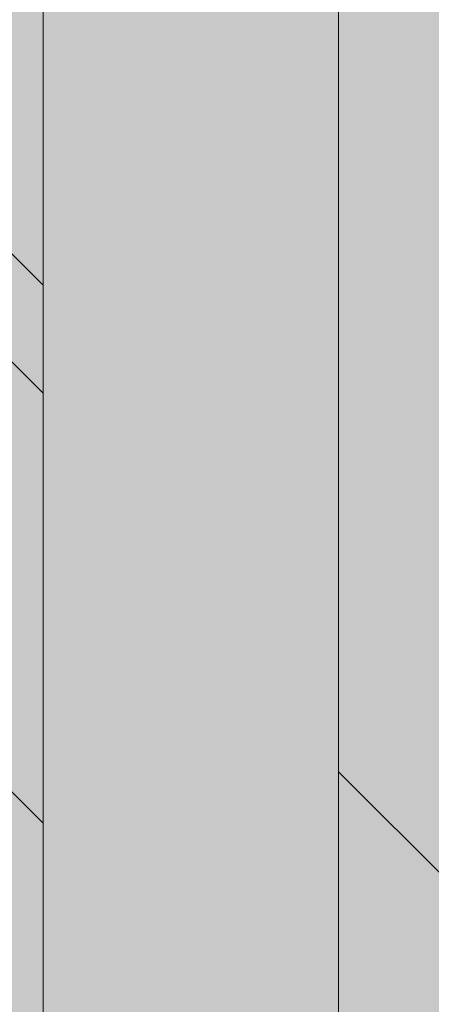
# Model space of a CAD drawing. Units: inches. Extents: x 844 to 2234, y 346 to 1084.
# Tile 38 of 93: x 1261.788 to 1262.676, y 699.229 to 701.353. Entities that reach past the tile are written whole.
import ezdxf

# ---------------------------------------------------------------- set-up
doc = ezdxf.new("R2010")
doc.units = ezdxf.units.IN
doc.header["$MEASUREMENT"] = 0
doc.layers.add('furniture', color=8, linetype='Continuous', lineweight=18)
doc.layers.add('RA-AP-01$0$INT', color=35, linetype='Continuous', lineweight=5)
doc.layers.add('RA-AP-01$0$FURN', color=3, linetype='Continuous')

# ---------------------------------------------------------------- blocks, each defined once
blk = doc.blocks.new('A$C18D01794')
at = {"layer": 'RA-AP-01$0$INT'}
h = blk.add_hatch(color=256, dxfattribs=at)
h.paths.add_polyline_path([(4.505206456958071, -7.585498806127123), (4.46934859260189, -7.549640941759413), (4.505206456958071, -7.513783077414768), (4.505206456958071, -7.381963272220687), (4.469348592616735, -7.346105407867824), (4.505206456958071, -7.310247543514964), (4.505206456958071, -7.178427738324996), (4.469348592586679, -7.142569873965138), (4.505206456952245, -7.106712009588038), (4.476922185709333, -7.106712009588038), (4.455206456960671, -7.128427738343681), (4.433490728198047, -7.106712009588038), (4.405206456946033, -7.106712009588036), (4.441064321339216, -7.142569873969684), (4.40520645695807, -7.178427738362358), (4.405206456958072, -7.310247543472698), (4.441064321364728, -7.346105407867826), (4.40520645695807, -7.381963272262947), (4.40520645695807, -7.513783077378263), (4.441064321354429, -7.549640941786153), (4.405206456958072, -7.585498806170974), (4.405206456958072, -7.717318611286652), (4.441064321333084, -7.753176475673194), (4.405206456958072, -7.789034340036673), (4.405206456958072, -8.006712009588039), (4.644348592588106, -8.006712009588039), (4.680206456964639, -7.970854145211967), (4.716064321341165, -8.006712009588039), (4.869348592586113, -8.006712009588039), (4.905206456964143, -7.970854145210465), (4.941064321342174, -8.006712009588039), (5.094348592587118, -8.006712009588037), (5.130206456963649, -7.970854145211967), (5.166064321340178, -8.006712009588039), (5.405206456958072, -8.006712009588039), (5.405206456958072, -7.789034340024526), (5.369348592595202, -7.753176475673196), (5.40520645695807, -7.717318611298797), (5.40520645695807, -7.585498806158829), (5.369348592573859, -7.549640941786151), (5.40520645695807, -7.51378307739041), (5.40520645695807, -7.381963272250803), (5.36934859256356, -7.346105407867824), (5.405206456958072, -7.310247543484846), (5.405206456958072, -7.178427738350217), (5.369348592589068, -7.142569873969682), (5.405206456982249, -7.106712009588038), (5.376922185730244, -7.106712009588038), (5.355206456967613, -7.128427738343679), (5.333490728218955, -7.10671200958804), (5.305206456976043, -7.106712009588042), (5.341064321341609, -7.142569873965136), (5.305206456958072, -7.178427738337141), (5.305206456958072, -7.310247543502816), (5.34106432131155, -7.346105407867824), (5.305206456958072, -7.381963272232832), (5.30520645695807, -7.513783077402624), (5.341064321326395, -7.549640941759413), (5.305206456958072, -7.585498806139263), (5.305206456958072, -7.717318611299605), (5.341064321347738, -7.753176475677737), (5.305206456958072, -7.78903434007894), (5.30520645695807, -7.906712009588039), (5.166064321336834, -7.906712009588039), (5.130206456963647, -7.942569873961684), (5.094348592590464, -7.906712009588039), (4.941064321338827, -7.906712009588041), (4.905206456964145, -7.942569873963183), (4.869348592589459, -7.906712009588039), (4.716064321337822, -7.906712009588041), (4.680206456964641, -7.942569873961684), (4.644348592591453, -7.906712009588039), (4.505206456958071, -7.906712009588039), (4.505206456958071, -7.789034340066795), (4.469348592580545, -7.753176475677738), (4.505206456958071, -7.717318611311748)])
h.paths.add_polyline_path([(4.485206456974132, -7.709034340046354), (4.45520645695909, -7.739034340051736), (4.425206456974128, -7.709034340057131), (4.425206456993394, -7.593783077384998), (4.45520645699153, -7.563783077396511), (4.485206456993396, -7.593783077408017)], flags=16)
h.paths.add_polyline_path([(4.455206456954537, -7.767318611299197), (4.485206456958242, -7.797318611312542), (4.48520645695951, -7.912569873958716), (4.45520645695415, -7.942569873954422), (4.425206456957888, -7.912569873967813), (4.425206456957888, -7.797318611286197)], flags=16)
h.paths.add_polyline_path([(4.455206456964794, -7.535498806149051), (4.42520645696469, -7.5054988061393), (4.425206456983954, -7.390247543486406), (4.455206456990734, -7.360247543489279), (4.485206456983953, -7.39024754349214), (4.485206456964687, -7.505498806158811)], flags=16)
h.paths.add_polyline_path([(4.499348592588947, -7.926712009585049), (4.636064321340932, -7.926712009585049), (4.666064321342317, -7.956712009586821), (4.636064321343707, -7.986712009585048), (4.499348592575121, -7.986712009585048), (4.469348592591685, -7.956712009591957)], flags=16)
h.paths.add_polyline_path([(4.425206456957888, -7.940854145195974), (4.471064321332215, -7.986712009585049), (4.425206456957888, -7.986712009585049)], flags=16)
h.paths.add_polyline_path([(4.455206456990734, -7.331963272246367), (4.425206456989053, -7.301963272254337), (4.425206456969784, -7.186712009596224), (4.455206456965226, -7.156712009591144), (4.485206456969787, -7.186712009586051), (4.485206456989053, -7.301963272238404)], flags=16)
h.paths.add_polyline_path([(4.72434859258714, -7.926712009586255), (4.861064321340141, -7.926712009586248), (4.891064321340324, -7.956712009586823), (4.861064321340513, -7.986712009586252), (4.724348592586768, -7.986712009586252), (4.694348592586956, -7.956712009586821)], flags=16)
h.paths.add_polyline_path([(4.919348592587961, -7.956712009586821), (4.949348592588145, -7.92671200958625), (5.08606432134115, -7.926712009586253), (5.116064321341327, -7.956712009586823), (5.086064321341519, -7.986712009586252), (4.949348592587774, -7.986712009586252)], flags=16)
h.paths.add_polyline_path([(5.144348592585967, -7.956712009586823), (5.174348592587358, -7.926712009585049), (5.311064321339338, -7.926712009585049), (5.3410643213366, -7.956712009591957), (5.311064321353163, -7.986712009585048), (5.174348592584576, -7.986712009585048)], flags=16)
h.paths.add_polyline_path([(5.32520645693489, -7.593783077408021), (5.355206456936755, -7.563783077396511), (5.385206456934894, -7.593783077384998), (5.38520645695416, -7.709034340057128), (5.355206456969194, -7.739034340051736), (5.325206456954153, -7.709034340046352)], flags=16)
h.paths.add_polyline_path([(5.325206456970042, -7.797318611312542), (5.355206456973747, -7.767318611299197), (5.385206456970398, -7.7973186112862), (5.385206456970398, -7.912569873967816), (5.355206456974136, -7.942569873954422), (5.325206456968778, -7.912569873958716)], flags=16)
h.paths.add_polyline_path([(5.325206456963599, -7.505498806158811), (5.325206456944333, -7.39024754349214), (5.355206456937552, -7.360247543489279), (5.385206456944332, -7.39024754348641), (5.385206456963596, -7.505498806139303), (5.355206456963492, -7.53549880614905)], flags=16)
h.paths.add_polyline_path([(5.32520645693923, -7.301963272238403), (5.3252064569585, -7.186712009586051), (5.355206456963062, -7.156712009591142), (5.3852064569585, -7.186712009596224), (5.385206456939234, -7.301963272254338), (5.355206456937552, -7.331963272246369)], flags=16)
h.paths.add_polyline_path([(5.339348592596071, -7.986712009585048), (5.385206456970398, -7.940854145195972), (5.385206456970396, -7.986712009585048)], flags=16)
h = blk.add_hatch(color=256, dxfattribs=at)
h.paths.add_polyline_path([(4.469348592586677, -7.142569873965136), (4.505206456958073, -7.178427738324996), (4.505206456958071, -7.106712009582215)])
h.paths.add_polyline_path([(4.455206456960671, -7.128427738343681), (4.476922185709333, -7.106712009588038), (4.433490728198045, -7.106712009588038)])
h.paths.add_polyline_path([(4.405206456958073, -7.178427738362358), (4.441064321339218, -7.142569873969684), (4.40520645695807, -7.106712009600073)])
h.paths.add_polyline_path([(4.425206456989053, -7.301963272254335), (4.455206456990736, -7.331963272246371), (4.485206456989055, -7.301963272238399), (4.48520645696979, -7.186712009586054), (4.455206456965227, -7.15671200959114), (4.425206456969784, -7.186712009596224)])
h.paths.add_polyline_path([(4.505206456958073, -7.381963272220689), (4.505206456958071, -7.310247543514961), (4.469348592616738, -7.346105407867826)])
h.paths.add_polyline_path([(4.425206456964688, -7.5054988061393), (4.455206456964794, -7.535498806149051), (4.485206456964689, -7.505498806158811), (4.485206456983951, -7.390247543492138), (4.455206456990736, -7.360247543489277), (4.425206456983956, -7.39024754348641)])
h.paths.add_polyline_path([(4.425206456974126, -7.709034340057128), (4.455206456959092, -7.739034340051736), (4.485206456974132, -7.709034340046356), (4.485206456993396, -7.593783077408017), (4.45520645699153, -7.563783077396511), (4.425206456993394, -7.593783077384999)])
h.paths.add_polyline_path([(4.46934859260189, -7.549640941759415), (4.505206456958071, -7.585498806127123), (4.505206456958073, -7.513783077414766)])
h.paths.add_polyline_path([(4.405206456958073, -7.585498806170972), (4.441064321354427, -7.549640941786151), (4.405206456958072, -7.513783077378263)])
h.paths.add_polyline_path([(4.405206456958072, -7.789034340036673), (4.441064321333084, -7.753176475673194), (4.405206456958072, -7.71731861128665)])
h.paths.add_polyline_path([(4.469348592580547, -7.75317647567774), (4.505206456958071, -7.789034340066795), (4.505206456958071, -7.717318611311744)])
h.paths.add_polyline_path([(4.425206456957888, -7.912569873967814), (4.45520645695415, -7.942569873954422), (4.485206456959507, -7.912569873958718), (4.48520645695824, -7.797318611312542), (4.455206456954537, -7.767318611299197), (4.425206456957888, -7.797318611286202)])
h.paths.add_polyline_path([(4.425206456957888, -7.986712009585049), (4.471064321332215, -7.986712009585049), (4.425206456957888, -7.940854145195972)])
h.paths.add_polyline_path([(4.499348592575121, -7.986712009585048), (4.636064321343707, -7.986712009585049), (4.666064321342317, -7.956712009586823), (4.636064321340932, -7.926712009585049), (4.499348592588945, -7.926712009585049), (4.469348592591685, -7.95671200959196)])
h.paths.add_polyline_path([(4.680206456964641, -7.942569873961684), (4.716064321337824, -7.906712009588039), (4.644348592591454, -7.906712009588039)])
h.paths.add_polyline_path([(4.644348592588108, -8.006712009588039), (4.716064321341167, -8.006712009588039), (4.680206456964637, -7.970854145211964)])
h.paths.add_polyline_path([(4.724348592586768, -7.98671200958625), (4.861064321340514, -7.986712009586252), (4.891064321340324, -7.956712009586819), (4.861064321340141, -7.92671200958625), (4.724348592587134, -7.926712009586255), (4.694348592586957, -7.956712009586821)])
h.paths.add_polyline_path([(4.905206456964143, -7.942569873963183), (4.941064321338827, -7.906712009588039), (4.869348592589457, -7.906712009588037)])
h.paths.add_polyline_path([(4.869348592586113, -8.006712009588039), (4.941064321342172, -8.006712009588037), (4.905206456964145, -7.970854145210463)])
h.paths.add_polyline_path([(4.949348592587774, -7.986712009586252), (5.086064321341521, -7.986712009586252), (5.116064321341329, -7.956712009586823), (5.08606432134115, -7.926712009586253), (4.949348592588145, -7.92671200958625), (4.919348592587961, -7.956712009586819)])
h.paths.add_polyline_path([(5.130206456963645, -7.942569873961684), (5.166064321336834, -7.906712009588039), (5.094348592590464, -7.906712009588039)])
h.paths.add_polyline_path([(5.094348592587119, -8.006712009588039), (5.166064321340178, -8.006712009588039), (5.130206456963651, -7.970854145211967)])
h.paths.add_polyline_path([(5.174348592584578, -7.986712009585048), (5.311064321353163, -7.986712009585048), (5.341064321336602, -7.956712009591958), (5.31106432133934, -7.926712009585049), (5.174348592587352, -7.926712009585049), (5.144348592585969, -7.956712009586823)])
h.paths.add_polyline_path([(5.325206456968778, -7.912569873958718), (5.355206456974136, -7.942569873954422), (5.385206456970396, -7.912569873967814), (5.385206456970396, -7.797318611286199), (5.355206456973747, -7.767318611299197), (5.325206456970044, -7.797318611312544)])
h.paths.add_polyline_path([(5.339348592596073, -7.986712009585048), (5.385206456970396, -7.986712009585049), (5.385206456970398, -7.94085414519597)])
h.paths.add_polyline_path([(5.325206456954155, -7.709034340046354), (5.355206456969194, -7.739034340051734), (5.38520645695416, -7.709034340057128), (5.385206456934896, -7.593783077384999), (5.355206456936758, -7.563783077396513), (5.325206456934888, -7.593783077408019)])
h.paths.add_polyline_path([(5.305206456958072, -7.789034340078938), (5.341064321347739, -7.753176475677738), (5.305206456958072, -7.717318611299605)])
h.paths.add_polyline_path([(5.369348592595204, -7.753176475673194), (5.40520645695807, -7.789034340024526), (5.405206456958072, -7.717318611298798)])
h.paths.add_polyline_path([(5.405206456958072, -7.585498806158831), (5.405206456958072, -7.513783077390407), (5.369348592573857, -7.549640941786151)])
h.paths.add_polyline_path([(5.305206456958072, -7.585498806139266), (5.341064321326393, -7.549640941759413), (5.305206456958072, -7.513783077402626)])
h.paths.add_polyline_path([(5.325206456963599, -7.50549880615881), (5.355206456963494, -7.535498806149055), (5.385206456963598, -7.505498806139302), (5.385206456944334, -7.390247543486411), (5.355206456937552, -7.360247543489279), (5.325206456944333, -7.39024754349214)])
h.paths.add_polyline_path([(5.305206456958072, -7.38196327223283), (5.341064321311551, -7.346105407867824), (5.305206456958072, -7.31024754350282)])
h.paths.add_polyline_path([(5.325206456939231, -7.301963272238404), (5.355206456937552, -7.331963272246369), (5.385206456939235, -7.301963272254335), (5.385206456958502, -7.186712009596224), (5.355206456963061, -7.156712009591142), (5.3252064569585, -7.186712009586051)])
h.paths.add_polyline_path([(5.404581768715993, -7.381338584008926, -0.001217816984214), (5.405206456958072, -7.381112009582329), (5.405206456958072, -7.310247543484846), (5.369348592563558, -7.346105407867826)])
h.paths.add_polyline_path([(5.36934859258907, -7.142569873969684), (5.40520645695807, -7.178427738350215), (5.405206456958072, -7.106712009612218)])
h.paths.add_polyline_path([(5.355206456967613, -7.128427738343683), (5.376922185730239, -7.106712009588038), (5.333490728218953, -7.10671200958804)])
h.paths.add_polyline_path([(5.30520645695807, -7.178427738337139), (5.341064321341609, -7.142569873965134), (5.305206456958074, -7.10671200957007)])
blk.add_hatch(color=256, dxfattribs=at).paths.add_polyline_path([(4.505206456958071, -7.906712009588039), (5.305206456958072, -7.906712009588039), (5.305206456958072, -7.106712009588038), (5.255206456951893, -7.106712009588036), (5.25520645694868, -7.856712009570104), (4.555206456959269, -7.856712009588616), (4.555206456956052, -7.106712009588038), (4.505206456958073, -7.106712009588038)])
h = blk.add_hatch(color=256, dxfattribs=at)
h.paths.add_polyline_path([(4.585917135068448, -7.856712009587804), (4.614201406330596, -7.856712009587056), (4.668846067270487, -7.802067348644738), (4.723490728212344, -7.856712009584164), (4.771774999457151, -7.856712009582887), (4.826419660396886, -7.80206734864072), (4.862780050090322, -7.838427738332541), (4.844495778842715, -7.856712009580965), (4.862780050090411, -7.856712009580482), (4.905206456960182, -7.814285602707865), (4.947632863832445, -7.856712009578238), (4.965917135079675, -7.856712009577755), (4.947632863831759, -7.838427738330656), (4.983993253523576, -7.802067348637219), (5.038637914464627, -7.856712009575829), (5.08692218571208, -7.856712009574554), (5.141566846649976, -7.802067348634224), (5.196211507589851, -7.856712009571666), (5.224495778822615, -7.856712009570916), (4.905206456953975, -7.537422687702283)])
h.paths.add_polyline_path([(4.895206456956031, -7.575706958950402), (4.895206456958921, -7.684996280828174), (4.840561796018589, -7.630351619890275)], flags=16)
h.paths.add_polyline_path([(4.915206456955638, -7.575706958949956), (4.969851117895509, -7.630351619887399), (4.915206456957609, -7.684996280827732)], flags=16)
h.paths.add_polyline_path([(4.826419660395175, -7.644493755514321), (4.881064321335613, -7.699138416452331), (4.771774999456703, -7.69913841645522)], flags=16)
h.paths.add_polyline_path([(4.983993253519558, -7.644493755510815), (5.038637914460456, -7.699138416449285), (4.929348592581548, -7.69913841645126)], flags=16)
h.paths.add_polyline_path([(4.881064321336025, -7.719138416452334), (4.826419660397532, -7.773783077393256), (4.771774999457062, -7.719138416455217)], flags=16)
h.paths.add_polyline_path([(4.929348592582019, -7.71913841645126), (5.038637914460982, -7.719138416449284), (4.983993253522945, -7.773783077389749)], flags=16)
h.paths.add_polyline_path([(4.895206456960191, -7.733280552075633), (4.895206456962115, -7.806001331460164), (4.876922185715016, -7.824285602708492), (4.840561796021581, -7.787925213016675)], flags=16)
h.paths.add_polyline_path([(4.915206456958487, -7.733280552075187), (4.969851117899527, -7.787925213013798), (4.933490728206909, -7.824285602708034), (4.9152064569598, -7.806001331461736)], flags=16)
h.paths.add_polyline_path([(4.757632863832376, -7.733280552079264), (4.812277524772842, -7.787925213017304), (4.757632863834348, -7.842569873958233)], flags=16)
h.paths.add_polyline_path([(4.737632863832376, -7.73328055207979), (4.737632863834348, -7.842569873958701), (4.682988202893906, -7.787925213020692)], flags=16)
h.paths.add_polyline_path([(5.05278005008503, -7.733280552072701), (5.052780050087917, -7.842569873951664), (4.998135389146995, -7.787925213013169)], flags=16)
h.paths.add_polyline_path([(5.072780050085024, -7.733280552072333), (5.127424711025931, -7.787925213010806), (5.072780050087916, -7.842569873951244)], flags=16)
h.paths.add_polyline_path([(4.935917135072783, -7.506712009583784), (5.255206456948811, -7.826001331459767), (5.255206456948932, -7.797717060211899), (5.200561796010279, -7.743072399273238), (5.255206456949403, -7.688427738334128), (5.25520645694961, -7.640143467086677), (5.200561796009787, -7.585498806146837), (5.236922185702417, -7.549138416454212), (5.255206456949919, -7.56742268770172), (5.255206456949998, -7.549138416454178), (5.212780050078687, -7.506712009583814), (5.25520645695036, -7.464285602712145), (5.255206456950438, -7.446001331464763), (5.236922185702424, -7.464285602712779), (5.200561796009796, -7.427925213020149), (5.255206456950753, -7.373280552079203), (5.25520645695096, -7.324996280834394), (5.200561796010322, -7.270351619893748), (5.255206456951428, -7.215706958952649), (5.255206456951547, -7.187422687705071)])
h.paths.add_polyline_path([(5.042988202883395, -7.42792521302065), (5.097632863823085, -7.373280552080975), (5.097632863822622, -7.482569873959883)], flags=16)
h.paths.add_polyline_path([(5.028846067259663, -7.442067348644384), (5.083490728198774, -7.496712009583504), (4.974201406321001, -7.496712009583035)], flags=16)
h.paths.add_polyline_path([(5.117632863823087, -7.37328055208089), (5.172277524762331, -7.42792521302015), (5.11763286382262, -7.482569873959851)], flags=16)
h.paths.add_polyline_path([(5.08349072819877, -7.516712009582191), (5.028846067259652, -7.571356670521302), (4.974201406320998, -7.516712009582638)], flags=16)
h.paths.add_polyline_path([(5.131774999446817, -7.35913841645716), (5.186419660386065, -7.413783077396415), (5.241064321325782, -7.359138416456712)], flags=17)
h.paths.add_polyline_path([(5.131774999446228, -7.496712009583703), (5.186419660386065, -7.442067348643883), (5.222780050079488, -7.478427738337313), (5.204495778832781, -7.496712009584014)], flags=16)
h.paths.add_polyline_path([(5.097632863822613, -7.530854145205813), (5.097632863823061, -7.640143467084723), (5.042988202883383, -7.585498806145032)], flags=16)
h.paths.add_polyline_path([(5.131774999446899, -7.339138416457162), (5.241064321325809, -7.339138416456712), (5.186419660386591, -7.284493755517479)], flags=17)
h.paths.add_polyline_path([(5.131774999446226, -7.516712009581999), (5.204495778830767, -7.516712009581702), (5.22278005007868, -7.534996280829206), (5.186419660386049, -7.571356670521828)], flags=16)
h.paths.add_polyline_path([(5.11763286382262, -7.530854145205852), (5.17227752476232, -7.585498806145562), (5.117632863823064, -7.64014346708481)], flags=16)
h.paths.add_polyline_path([(5.186419660386069, -7.599640941770585), (5.241064321325754, -7.654285602710281), (5.131774999446791, -7.654285602709814)], flags=16)
h.paths.add_polyline_path([(5.131774999446872, -7.674285602709813), (5.24106432132578, -7.674285602710282), (5.186419660386554, -7.728930263649504)], flags=16)
h.paths.add_polyline_path([(5.255206456951811, -7.126001331467467), (5.255206456951895, -7.106712009588038), (4.555206456956052, -7.106712009588038), (4.555206456956136, -7.12600133146746), (4.905206456953973, -7.476001331465289)])
h.paths.add_polyline_path([(4.983993253513404, -7.368930263651977), (4.92934859257295, -7.314285602713969), (5.03863791445186, -7.314285602711063)], flags=16)
h.paths.add_polyline_path([(4.969851117889988, -7.383072399276016), (4.915206456952556, -7.437717060215906), (4.915206456949648, -7.328427738338133)], flags=16)
h.paths.add_polyline_path([(4.929348592572535, -7.294285602713971), (4.983993253511019, -7.239640941773039), (5.038637914451496, -7.294285602711065)], flags=16)
h.paths.add_polyline_path([(5.052780050074912, -7.280143467087016), (4.998135389134438, -7.225498806148989), (5.052780050072919, -7.170854145208052)], flags=16)
h.paths.add_polyline_path([(5.07278005007491, -7.280143467086489), (5.072780050072918, -7.170854145207579), (5.127424711013374, -7.225498806145578)], flags=16)
h.paths.add_polyline_path([(4.89520645695295, -7.437717060216355), (4.840561796013067, -7.383072399278919), (4.895206456950961, -7.328427738338582)], flags=16)
h.paths.add_polyline_path([(4.915206456948365, -7.280143467090674), (4.915206456946434, -7.207422687704125), (4.933490728192729, -7.18913841645701), (4.969851117886972, -7.225498806149623)], flags=16)
h.paths.add_polyline_path([(4.881064321327021, -7.314285602715054), (4.82641966038902, -7.368930263655506), (4.771774999448108, -7.314285602717047)], flags=16)
h.paths.add_polyline_path([(4.895206456950073, -7.280143467091125), (4.840561796009022, -7.225498806152518), (4.876922185700835, -7.18913841645908), (4.895206456948749, -7.207422687706589)], flags=16)
h.paths.add_polyline_path([(4.983993253510392, -7.211356670525576), (4.947632863816944, -7.174996280833758), (4.965917135064043, -7.156712009585847), (5.038637914448995, -7.156712009584522)], flags=16)
h.paths.add_polyline_path([(4.881064321326543, -7.294285602715056), (4.771774999447578, -7.294285602717046), (4.826419660385607, -7.239640941776569)], flags=16)
h.paths.add_polyline_path([(4.905206456946447, -7.19913841645844), (4.862780050074785, -7.156712009587725), (4.947632863816685, -7.156712009586302)], flags=16)
h.paths.add_polyline_path([(5.14156684663679, -7.211356670521528), (5.086922185696452, -7.156712009583639), (5.196211507574223, -7.156712009581651)], flags=16)
h.paths.add_polyline_path([(4.8264196603837, -7.211356670529104), (4.771774999442643, -7.156712009590501), (4.8444957788276, -7.156712009588568), (4.862780050075511, -7.17499628083566)], flags=16)
h.paths.add_polyline_path([(4.812277524760289, -7.225498806153156), (4.757632863822258, -7.28014346709363), (4.757632863819352, -7.170854145214669)], flags=16)
h.paths.add_polyline_path([(4.73763286382226, -7.280143467093997), (4.682988202881349, -7.22549880615554), (4.737632863819352, -7.170854145215086)], flags=16)
h.paths.add_polyline_path([(4.723490728195188, -7.156712009591787), (4.668846067257299, -7.211356670532127), (4.614201406317417, -7.156712009594693)], flags=16)
h.paths.add_polyline_path([(4.597632863829262, -7.506712009583814), (4.555206456957951, -7.54913841645418), (4.555206456958029, -7.56742268770172), (4.573490728205535, -7.549138416454212), (4.609851117898167, -7.585498806146839), (4.555206456958338, -7.640143467086675), (4.555206456958546, -7.688427738334125), (4.60985111789767, -7.743072399273238), (4.555206456959015, -7.797717060211899), (4.555206456959138, -7.826001331459767), (4.874495778835167, -7.506712009583786), (4.5552064569564, -7.187422687705062), (4.555206456956523, -7.215706958952644), (4.609851117897629, -7.270351619893746), (4.555206456956988, -7.324996280834396), (4.555206456957198, -7.373280552079195), (4.609851117898153, -7.427925213020147), (4.573490728205528, -7.464285602712779), (4.555206456957507, -7.446001331464756), (4.555206456957585, -7.464285602712143)])
h.paths.add_polyline_path([(4.712780050085332, -7.482569873959882), (4.712780050084863, -7.373280552080972), (4.767424711024555, -7.42792521302065)], flags=16)
h.paths.add_polyline_path([(4.726922185709173, -7.496712009583504), (4.781566846648288, -7.442067348644384), (4.836211507586949, -7.496712009583033)], flags=16)
h.paths.add_polyline_path([(4.692780050085327, -7.482569873959851), (4.638135389145619, -7.427925213020149), (4.692780050084865, -7.373280552080892)], flags=16)
h.paths.add_polyline_path([(4.726922185709182, -7.516712009582191), (4.836211507586949, -7.51671200958264), (4.7815668466483, -7.571356670521304)], flags=16)
h.paths.add_polyline_path([(4.678637914461726, -7.496712009583706), (4.605917135075169, -7.496712009584014), (4.587632863828464, -7.478427738337311), (4.623993253521887, -7.442067348643881)], flags=16)
h.paths.add_polyline_path([(4.712780050085336, -7.530854145205816), (4.767424711024568, -7.585498806145034), (4.71278005008489, -7.640143467084724)], flags=16)
h.paths.add_polyline_path([(4.678637914461726, -7.516712009582001), (4.623993253521899, -7.571356670521829), (4.587632863829271, -7.534996280829206), (4.605917135077185, -7.5167120095817)], flags=16)
h.paths.add_polyline_path([(4.692780050085336, -7.530854145205848), (4.692780050084889, -7.64014346708481), (4.638135389145632, -7.585498806145562)], flags=16)
h.paths.add_polyline_path([(4.623993253521885, -7.413783077396415), (4.678637914461131, -7.359138416457161), (4.56934859258217, -7.359138416456712)], flags=17)
h.paths.add_polyline_path([(4.623993253521901, -7.599640941770568), (4.678637914461158, -7.654285602709814), (4.569348592582195, -7.654285602710281)], flags=16)
h.paths.add_polyline_path([(4.678637914461051, -7.339138416457162), (4.623993253521361, -7.284493755517479), (4.569348592582143, -7.339138416456712)], flags=17)
h.paths.add_polyline_path([(4.678637914461076, -7.674285602709813), (4.623993253521399, -7.728930263649504), (4.569348592582167, -7.674285602710281)], flags=16)
h = blk.add_hatch(color=256, dxfattribs=at)
h.paths.add_polyline_path([(4.781566846647504, -7.442067348645805), (4.836211507586161, -7.496712009584463), (4.726922185708388, -7.496712009584918)])
h.paths.add_polyline_path([(4.836211507586161, -7.516712009584068), (4.781566846647504, -7.571356670522723), (4.726922185708388, -7.516712009583606)])
h.paths.add_polyline_path([(4.76742471102377, -7.585498806146453), (4.712780050084083, -7.640143467086137), (4.712780050084542, -7.530854145207227)])
h.paths.add_polyline_path([(4.692780050084544, -7.530854145207257), (4.692780050084084, -7.64014346708622), (4.638135389144834, -7.585498806146965)])
h.paths.add_polyline_path([(4.678637914460932, -7.516712009583407), (4.623993253521102, -7.571356670523233), (4.587632863827676, -7.53499628082981), (4.605917135074382, -7.516712009583104)])
h.paths.add_polyline_path([(4.573490728204743, -7.54913841645434), (4.60985111789737, -7.585498806146969), (4.555206456957541, -7.640143467086797), (4.555206456957237, -7.567422687701846)])
h.paths.add_polyline_path([(4.623993253521098, -7.599640941770699), (4.67863791446035, -7.654285602709951), (4.56934859258139, -7.654285602710407)])
h.paths.add_polyline_path([(4.678637914460275, -7.67428560270995), (4.623993253520583, -7.728930263649637), (4.56934859258136, -7.674285602710405)])
h.paths.add_polyline_path([(4.609851117896854, -7.743072399273369), (4.555206456958196, -7.797717060212026), (4.555206456957738, -7.688427738334254)])
h.paths.add_polyline_path([(4.597632863828475, -7.506712009583301), (4.555206456957283, -7.549138416454495), (4.555206456956805, -7.464285602712587)])
h.paths.add_polyline_path([(4.678637914460932, -7.496712009585113), (4.605917135076396, -7.496712009585417), (4.587632863828479, -7.478427738337913), (4.623993253521104, -7.442067348645284)])
h.paths.add_polyline_path([(4.692780050084091, -7.373280552082301), (4.692780050084548, -7.482569873961267), (4.638135389144834, -7.427925213021552)])
h.paths.add_polyline_path([(4.767424711023772, -7.427925213022072), (4.712780050084545, -7.48256987396129), (4.712780050084089, -7.373280552082384)])
h.paths.add_polyline_path([(4.67863791446036, -7.359138416457298), (4.623993253521105, -7.41378307739655), (4.569348592581399, -7.35913841645684)])
h.paths.add_polyline_path([(4.609851117897371, -7.427925213020278), (4.573490728204743, -7.464285602712907), (4.555206456957237, -7.446001331465401), (4.555206456957548, -7.373280552080448)])
h.paths.add_polyline_path([(4.623993253520596, -7.284493755517612), (4.67863791446028, -7.339138416457299), (4.569348592581367, -7.339138416456838)])
h.paths.add_polyline_path([(4.609851117896867, -7.270351619893878), (4.555206456957749, -7.324996280832994), (4.55520645695821, -7.21570695895522)])
for p, q in [((4.555206456956052, -7.106712009588036), (4.555206456959269, -7.856712009588616)), ((4.505206456987672, -7.381963272250288), (4.469348592616737, -7.346105407867824)), ((4.555206456958024, -7.446001331465273), (4.555206456958322, -7.373280552080322)), ((4.555206456958322, -7.373280552080322), (4.609851117898155, -7.427925213020149)), ((4.555206456958022, -7.446001331465273), (4.573490728205528, -7.464285602712781)), ((4.573490728205528, -7.464285602712779), (4.55520645695807, -7.446001331465319)), ((4.597632863829264, -7.506712009583814), (4.55520645695807, -7.464285602712626)), ((4.55520645695807, -7.464285602712626), (4.555206456957598, -7.549138416454534))]:
    blk.add_line(p, q, dxfattribs=at)
blk.add_lwpolyline([(5.305206456958072, -7.106712009588038), (5.305206456958072, -7.906712009588039), (4.505206456958071, -7.906712009588039), (4.505206456958071, -7.106712009588038)], dxfattribs=at)
blk = doc.blocks.new('A$C5D2F253E')
at = {"layer": 'RA-AP-01$0$FURN', "xscale": -0.7999999999883585, "yscale": 0.7999999999883585, "zscale": 0.8, "rotation": 90}
blk.add_blockref('A$C18D01794', (-5.687757199772477, 4.75791982714071), dxfattribs=at)

msp = doc.modelspace()

# ---------------------------------------------------------------- block references
at = {"layer": 'furniture', "xscale": -15.94108302203742, "yscale": 15.94108302203742, "zscale": 15.94108302203742, "rotation": 270}
msp.add_blockref('A$C5D2F253E', (1244.08405109492, 696.2584716700112), dxfattribs=at)

doc.saveas('drawing.dxf')
